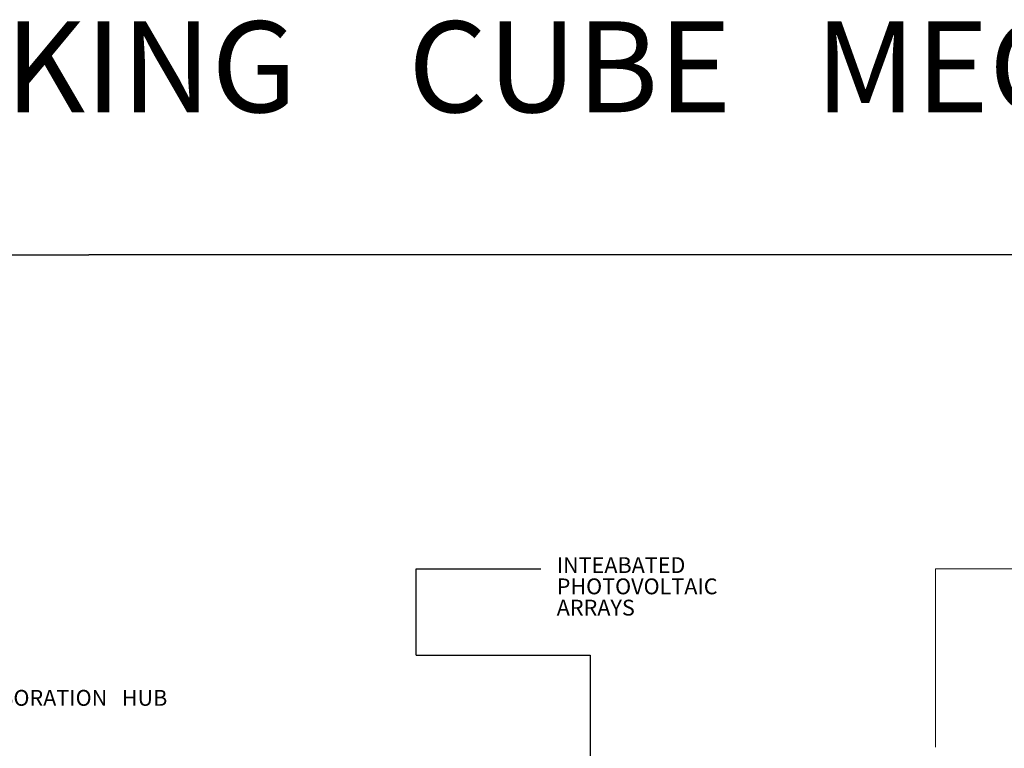
# Model space of a CAD drawing. Units: inches. Extents: x -32109 to 33221, y -19197 to 7608.
# Tile 17 of 25: x -741 to 6939, y 1922 to 7608. Entities that reach past the tile are written whole.
import ezdxf

# ---------------------------------------------------------------- set-up
doc = ezdxf.new("R2010")
doc.units = ezdxf.units.IN
doc.header["$MEASUREMENT"] = 0
for name, color, linetype, lineweight in [('A-ANNO-DIMS', 2, 'Continuous', 18), ('A-ANNO-NOTE', 2, 'Continuous', 18), ('A-ANNO-TEXT', 7, 'Continuous', 25), ('A-ELEV', 7, 'Continuous', 25)]:
    doc.layers.add(name, color=color, linetype=linetype, lineweight=lineweight)
doc.styles.get("Standard").update_dxf_attribs({"font": 'arial.ttf'})
doc.dimstyles.get("Standard").update_dxf_attribs({"dimtxt": 0.18, "dimasz": 0.18, "dimexe": 0.18, "dimexo": 0.0625, "dimgap": 0.09, "dimtad": 0, "dimtih": 1, "dimtoh": 1, "dimdec": 4, "dimzin": 0, "dimdsep": 46, "dimtxsty": 'Standard', "dimcen": 0.09, "dimadec": 0, "dimazin": 0, "dimtfac": 1, "dimtdec": 4, "dimtofl": 0, "dimtmove": 0, "dimatfit": 3, "dimfxl": 1, "dimtolj": 1, "dimtzin": 0, "dimarcsym": 0})

# ---------------------------------------------------------------- blocks, each defined once
blk = doc.blocks.new('*D10')
at = {"layer": 'A-ANNO-DIMS', "color": 0, "lineweight": -2, "transparency": 16777216}
for p, q in [((-18512.646816, -110.179138), (-18512.646816, 5772.015489000001)), ((-18512.466816, 5771.835489), (-202.0927503703958, 5771.835489)), ((18109.136745, 5771.835489), (-201.2373206296045, 5771.835489)), ((18109.316745, -101.537382), (18109.316745, 5772.015489000001))]:
    blk.add_line(p, q, dxfattribs=at)
at = {"layer": 'A-ANNO-DIMS', "color": 0, "transparency": 16777216}
for points in [[(-18512.466816, 5771.865488999999), (-18512.466816, 5771.805489000001), (-18512.646816, 5771.835489)], [(18109.136745, 5771.865488999999), (18109.136745, 5771.805489000001), (18109.316745, 5771.835489)]]:
    blk.add_solid(points, dxfattribs=at)
at = {"layer": 'Defpoints', "color": 0, "transparency": 16777216}
for p in [(18109.316745, 5771.835489), (-18512.646816, -110.241638), (18109.316745, -101.599882)]:
    blk.add_point(p, dxfattribs=at)
at = {"layer": 'A-ANNO-DIMS', "color": 0, "transparency": 16777216, "insert": (-201.6650355000002, 5771.835489), "char_height": 0.18, "attachment_point": 5}
blk.add_mtext('\\A1;36622', dxfattribs=at)

msp = doc.modelspace()

# ---------------------------------------------------------------- linework, layer by layer
at = {"layer": 'A-ANNO-NOTE'}
for p, q in [((6402.717398849782, 1930.74681286182), (6402.717398849883, 3321.835488633435)), ((6402.717398849883, 3321.835488633435), (7145.280624769163, 3321.835488633435))]:
    msp.add_line(p, q, dxfattribs=at)
at = {"layer": 'A-ELEV'}
for p, q in [((2351.113958139424, 3321.835488633431), (3323.745815389208, 3321.835488633431)), ((2351.113958139355, 2649.474070118566), (2351.113958139424, 3321.835488633431)), ((2351.113958139355, 2649.474070118566), (3709.007830620743, 2649.474070118566)), ((3709.007830620743, 2649.474070118566), (3709.007830620743, 1327.301250283199))]:
    msp.add_line(p, q, dxfattribs=at)

# ---------------------------------------------------------------- texts
at = {"layer": 'A-ANNO-TEXT'}
for s, height, p in [('COMPREHENSIVE   ARCHITECTURAL   INTERLOCKING    CUBE   MEGA   CAMPUC   MASTER   PLAN ', 709.7949465747753, (-22238.10681632875, 6885.298304043546)), ('INTEABATED ', 123.5547426012344, (3447.942543036188, 3289.825983001363)), ('PHOTOVOLTAIC', 123.5547426012344, (3447.942543036188, 3123.829766859861)), ('ARRAYS', 123.5547426012344, (3447.942543036188, 2957.833550718359)), ('CENTRALIZE    COLLABORATION   HUB', 123.5547426012344, (-2550.352267461713, 2253.722659563042))]:
    msp.add_text(s, height=height, dxfattribs=at).set_placement(p)

# ---------------------------------------------------------------- dimensions: what is measured, and where the dimension line sits
at = {"layer": 'A-ANNO-DIMS'}
dim = msp.add_linear_dim(base=(18109.316745, 5771.835489), p1=(-18512.646816, -110.241638), p2=(18109.316745, -101.599882), dimstyle='Standard', override={"dimdec": 0, "dimlfac": 1, "dimrnd": 0, "dimzin": 0, "dimdsep": 46, "dimlunit": 2}, dxfattribs=at)
dim.commit()
dim.dimension.update_dxf_attribs({"geometry": '*D10', "text_midpoint": (-201.6650355000002, 5771.835489)})

doc.saveas('drawing.dxf')
